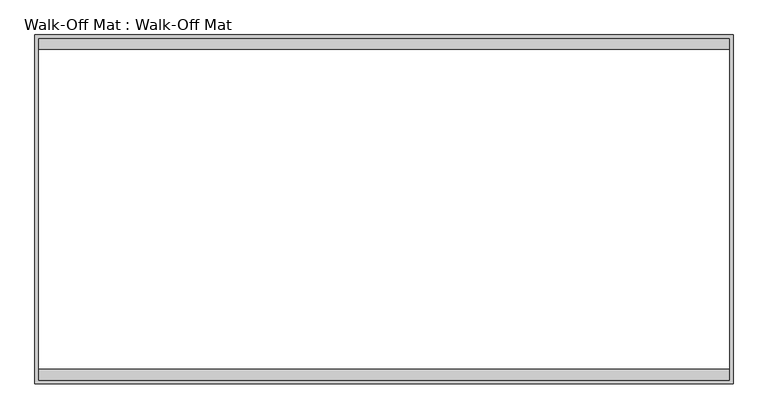
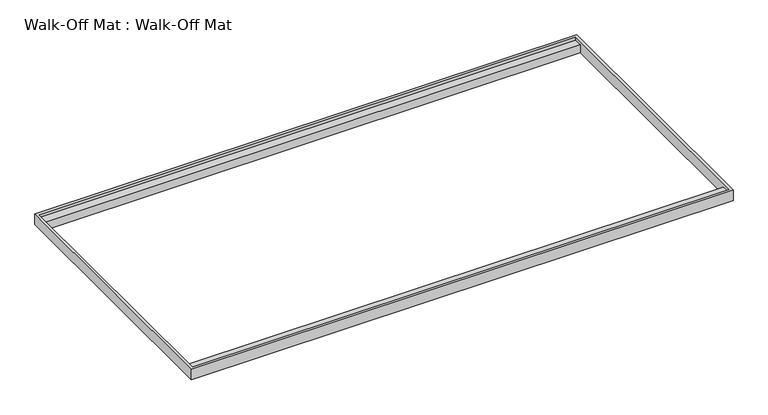
"""IFC4 building model written with IfcOpenShell, lengths in millimetres: proxy geometry, Walk-Off Mat : Walk-Off Mat."""

from ifc_helpers import new_model, si_unit, origin, place, context, project, spatial, faceted_brep, source, transform, mapped, element, save


def walk_off_mat_walk_off_mat_25c2b8c1(model_context):
    return source(origin(), model_context, "Body", "Brep", [
        faceted_brep([(209.8145383, -1047.7440671, 0.0), (209.8145383, -450.8440671, 0.0), (209.8145383, -450.8440671, -6.35), (209.8145383, -469.8940671, -6.35), (209.8145383, -469.8940671, -25.4), (209.8145383, -1028.6940671, -25.4), (209.8145383, -1028.6940671, -6.35), (209.8145383, -1047.7440671, -6.35), (216.1645383, -444.4940671, -25.4), (216.1645383, -444.4940671, 0.0), (216.1645383, -1054.0940671, 0.0), (216.1645383, -1054.0940671, -25.4), (-996.6854617, -1047.7440671, 0.0), (-996.6854617, -1047.7440671, -6.35), (-1003.0354617, -1054.0940671, 0.0), (-1003.0354617, -1054.0940671, -25.4), (-996.6854617, -450.8440671, 0.0), (-996.6854617, -1028.6940671, -6.35), (-996.6854617, -1028.6940671, -25.4), (-996.6854617, -469.8940671, -25.4), (-996.6854617, -469.8940671, -6.35), (-996.6854617, -450.8440671, -6.35), (-1003.0354617, -444.4940671, 0.0), (-1003.0354617, -444.4940671, -25.4)], [[[0, 1, 2, 3, 4, 5, 6, 7]], [[8, 9, 10, 11]], [[12, 0, 7, 13]], [[11, 10, 14, 15]], [[16, 12, 13, 17, 18, 19, 20, 21]], [[15, 14, 22, 23]], [[8, 11, 15, 23], [18, 5, 4, 19]], [[1, 16, 21, 2]], [[10, 9, 22, 14], [1, 0, 12, 16]], [[9, 8, 23, 22]], [[6, 17, 13, 7]], [[17, 6, 5, 18]], [[20, 3, 2, 21]], [[3, 20, 19, 4]]]),
    ])


if __name__ == "__main__":
    model = new_model("IFC4")
    model_context = context("Model", 3, world=origin())
    ifc_project = project(units=[si_unit("LENGTHUNIT", "METRE", prefix="MILLI")], contexts=[model_context])
    site = spatial("IfcSite", under=ifc_project)
    building = spatial("IfcBuilding", under=site)
    placement = place(None, origin())
    walk_off_mat_walk_off_mat_shape = walk_off_mat_walk_off_mat_25c2b8c1(model_context)
    element("IfcBuildingElementProxy", 1, Name="Walk-Off Mat : Walk-Off Mat", ObjectType="Walk-Off Mat : Walk-Off Mat", at=placement, inside=building, context=model_context, shape_type="MappedRepresentation", body=[
        mapped(walk_off_mat_walk_off_mat_shape, transform((0.0, 0.0, 0.0), x_axis=(1.0, 0.0, 0.0), y_axis=(0.0, 1.0, 0.0), z_axis=(0.0, 0.0, 1.0))),
    ])
    save(model, "model.ifc")

# Revit data of these elements
# Type "Walk-Off Mat : Walk-Off Mat"
#   Width [instance default] = 4' - 0"
#   Length [instance default] = 2' - 0"
#   Array Length [instance default] = 1' - 10"
#   WebArrayNum [instance default] = 18
#   Default Elevation = 0
# Element 1 (IfcBuildingElementProxy, "Walk-Off Mat : Walk-Off Mat")
#   Materials on its faces: "Aluminum"
# Materials
#   "Aluminum": class "Metal", colour RGB 247 247 247, transparency 0, Description = "Aluminum 6061", Cost = 0
